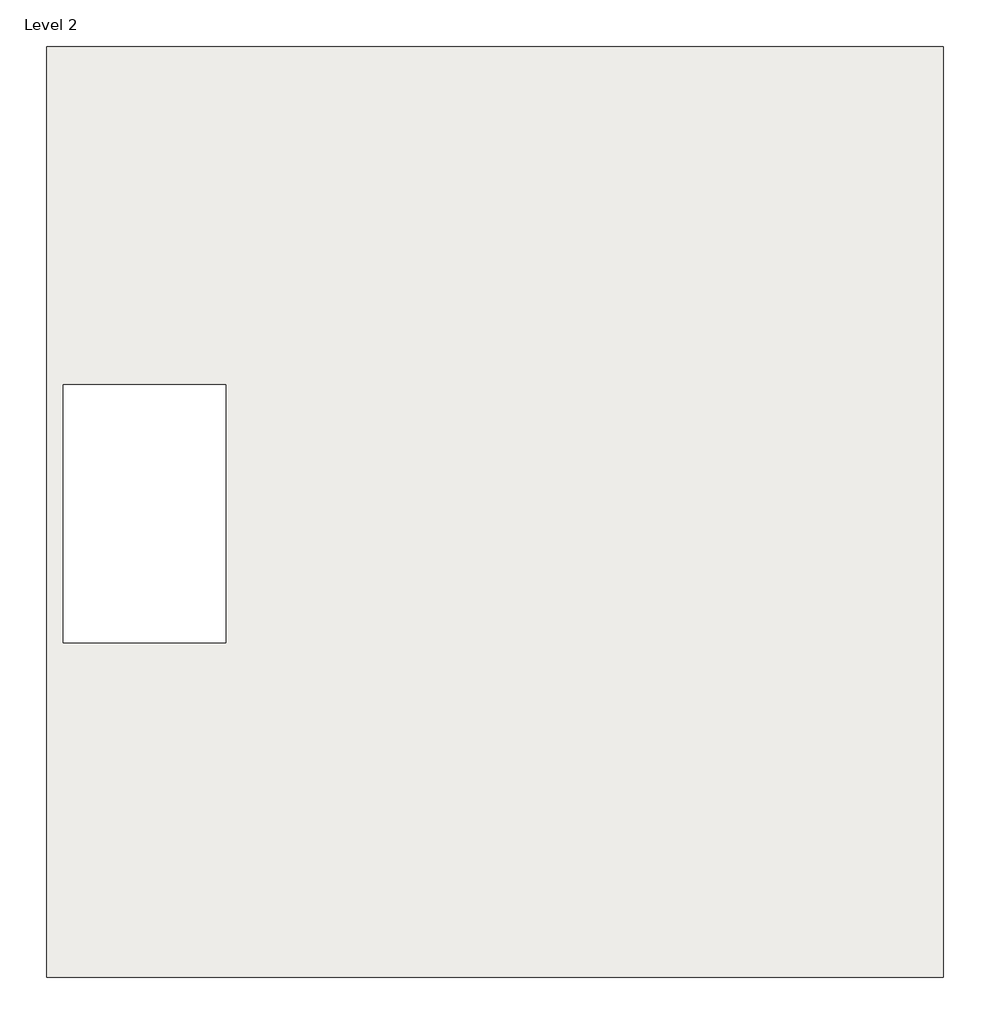
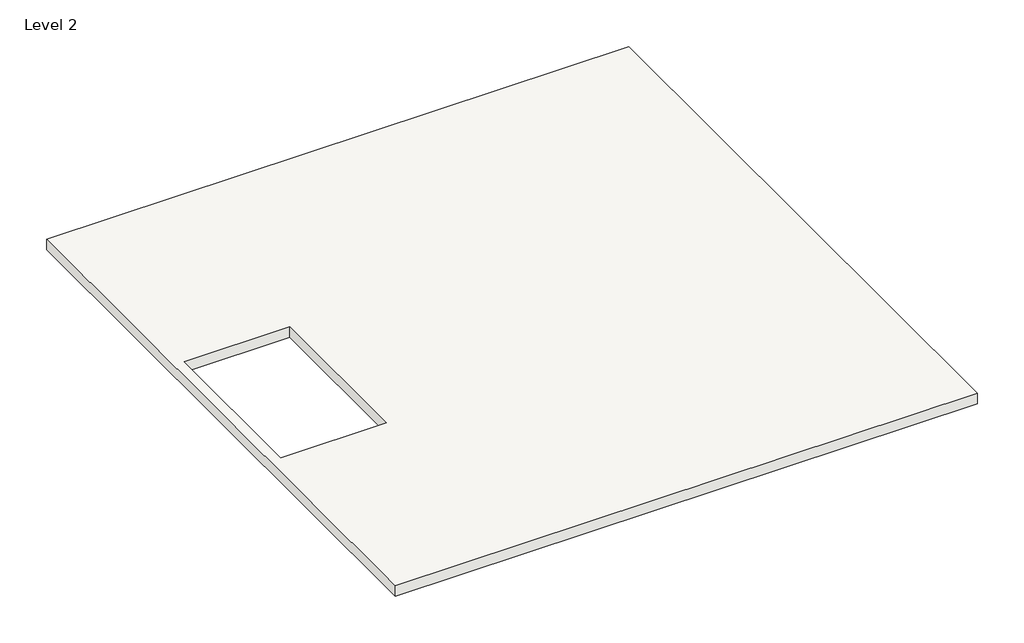
# One storey: 1 roof.
"""IFC4 building model written with IfcOpenShell, lengths in millimetres."""

from ifc_helpers import new_model, si_unit, frame, origin, place, context, project, spatial, polyline, outline, extrude, element, save

model = new_model("IFC4")

# Units and contexts
model_context = context("Model", 3, world=origin())
ifc_project = project(units=[si_unit("LENGTHUNIT", "METRE", prefix="MILLI")], contexts=[model_context])

# Site, building, storey
site = spatial("IfcSite", under=ifc_project)
building = spatial("IfcBuilding", under=site)
storey = spatial("IfcBuildingStorey", under=building, Name="Level 2", Elevation=3048.0)

# Roof
placement = place(None, origin())
element("IfcRoof", 1, ObjectType="Generic - 12\"", at=placement, inside=storey, context=model_context, shape_type="SweptSolid", body=[
    extrude(outline(polyline([(-15419.18283, 14812.8620171), (557.41717, 14812.8620171), (557.41717, -1773.3379829), (-15419.18283, -1773.3379829), (-15419.18283, 14812.8620171)]), holes=[polyline([(-12224.5393867, 4185.7990122), (-12224.5393867, 8783.1990122), (-15120.1393867, 8783.1990122), (-15120.1393867, 4185.7990122), (-12224.5393867, 4185.7990122)])]), frame((0.0, 0.0, 3048.0), z_axis=(0.0, 0.0, 1.0), x_axis=(1.0, 0.0, 0.0)), (0.0, 0.0, 1.0), 304.8),
])

save(model, "model.ifc")

# Revit data of these elements
# Type "Generic - 12\""
#   Assembly Code = "B1020"
#   Layers, outside or top first: 1' - 0" "Brick, Soldier Course" (function 1)
# Element 1 (IfcRoof, "Generic - 12\"")
#   built-in parameter 1001705 = 11 (stored number, unit not read)
#   built-in parameter 1001710 = 33615
#   Phase Created = New Construction
#   Materials on its faces: "Brick, Soldier Course"
# Materials
#   "Brick, Soldier Course": class "Masonry", colour RGB 170 98 104, transparency 0, Description = "Common brick soldier coursed", Cost = 0
